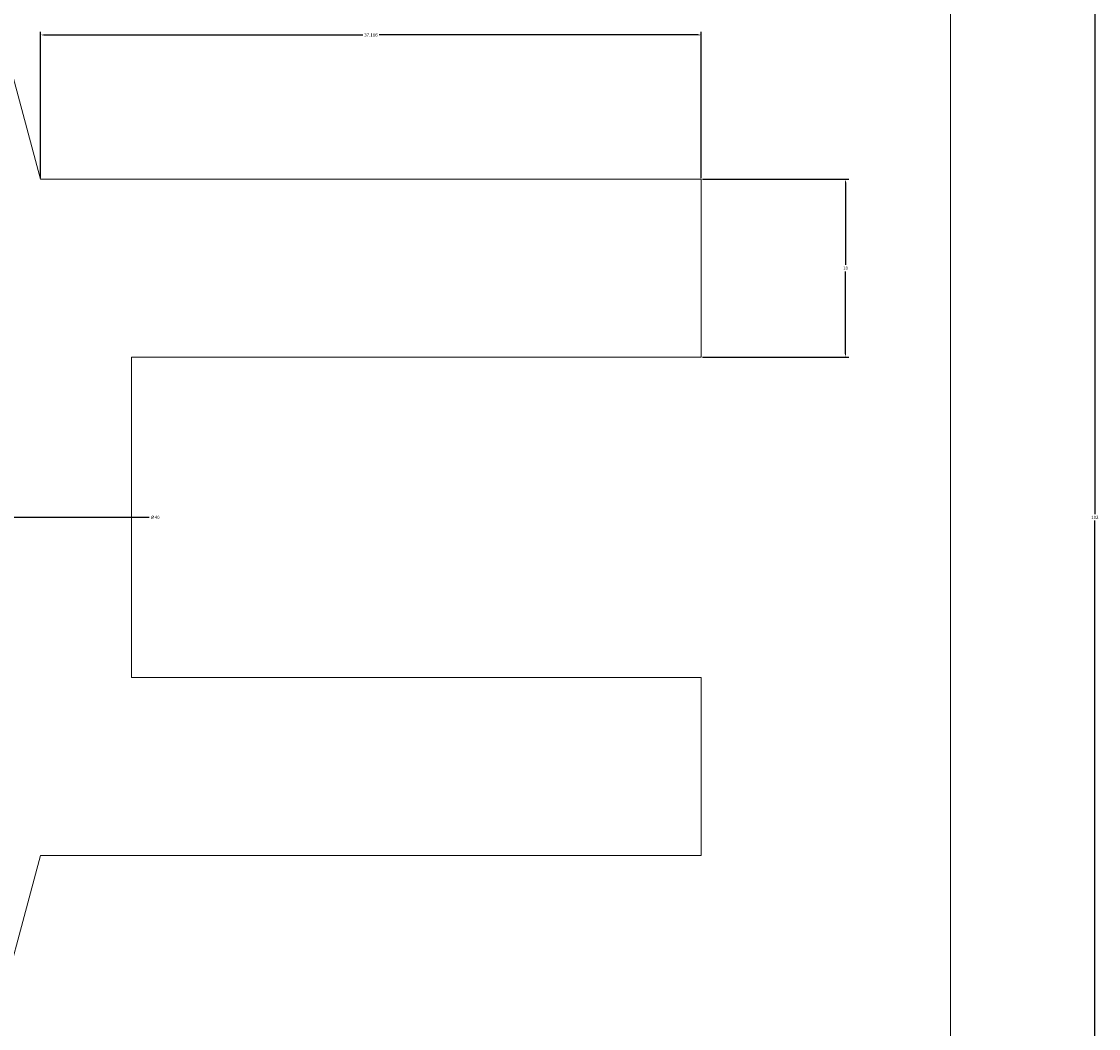
# Model space of a CAD drawing. Units: millimetres. Extents: x 2597 to 2768, y 1809 to 1980.
# Tile 6 of 7: x 2708 to 2768, y 1866 to 1922. Entities that reach past the tile are written whole.
import ezdxf

# ---------------------------------------------------------------- set-up
doc = ezdxf.new("R2010")
doc.units = ezdxf.units.MM
doc.layers.add('M-CONS', color=8, linetype='Continuous', lineweight=18)
doc.layers.add('M-DIMS', color=2, linetype='Continuous', lineweight=18)
doc.styles.get("Standard").update_dxf_attribs({"font": 'arial.ttf'})
doc.dimstyles.get("Standard").update_dxf_attribs({"dimtxt": 0.18, "dimasz": 0.18, "dimexe": 0.18, "dimexo": 0.0625, "dimgap": 0.09, "dimtad": 0, "dimtih": 1, "dimtoh": 1, "dimdec": 4, "dimzin": 0, "dimdsep": 46, "dimtxsty": 'Standard', "dimcen": 0.09, "dimadec": 0, "dimazin": 0, "dimtfac": 1, "dimtdec": 4, "dimtofl": 0, "dimtmove": 0, "dimatfit": 3, "dimfxl": 1, "dimtolj": 1, "dimtzin": 0, "dimarcsym": 0})

# ---------------------------------------------------------------- blocks, each defined once
blk = doc.blocks.new('*D6')
at = {"layer": 'Defpoints', "color": 0, "transparency": 16777216}
for p in [(2733.776, 1945.43), (2767.876, 1945.43), (2733.776, 1843.43)]:
    blk.add_point(p, dxfattribs=at)
at = {"layer": 'M-DIMS', "color": 0, "lineweight": -2, "transparency": 16777216}
for p, q in [((2733.838, 1945.43), (2768.056, 1945.43)), ((2767.876, 1945.25), (2767.876, 1894.612)), ((2767.876, 1843.61), (2767.876, 1894.248)), ((2733.838, 1843.43), (2768.056, 1843.43))]:
    blk.add_line(p, q, dxfattribs=at)
at = {"layer": 'M-DIMS', "color": 0, "transparency": 16777216}
for points in [[(2767.846, 1945.25), (2767.906, 1945.25), (2767.876, 1945.43)], [(2767.846, 1843.61), (2767.906, 1843.61), (2767.876, 1843.43)]]:
    blk.add_solid(points, dxfattribs=at)
at = {"layer": 'M-DIMS', "color": 0, "transparency": 16777216, "insert": (2767.876, 1894.43), "char_height": 0.18, "attachment_point": 5}
blk.add_mtext('\\A1;102', dxfattribs=at)
blk = doc.blocks.new('*D11')
at = {"layer": 'Defpoints', "color": 0, "transparency": 16777216}
for p in [(2745.776, 1913.43), (2745.776, 1903.43), (2753.876, 1903.43)]:
    blk.add_point(p, dxfattribs=at)
at = {"layer": 'M-DIMS', "color": 0, "lineweight": -2, "transparency": 16777216}
for p, q in [((2745.838, 1913.43), (2754.056, 1913.43)), ((2753.876, 1913.25), (2753.876, 1908.612)), ((2753.876, 1903.61), (2753.876, 1908.248)), ((2745.838, 1903.43), (2754.056, 1903.43))]:
    blk.add_line(p, q, dxfattribs=at)
at = {"layer": 'M-DIMS', "color": 0, "transparency": 16777216}
for points in [[(2753.846, 1913.25), (2753.906, 1913.25), (2753.876, 1913.43)], [(2753.846, 1903.61), (2753.906, 1903.61), (2753.876, 1903.43)]]:
    blk.add_solid(points, dxfattribs=at)
at = {"layer": 'M-DIMS', "color": 0, "transparency": 16777216, "insert": (2753.876, 1908.43), "char_height": 0.18, "attachment_point": 5}
blk.add_mtext('\\A1;10', dxfattribs=at)
blk = doc.blocks.new('*D12')
at = {"layer": 'Defpoints', "color": 0, "transparency": 16777216}
for p in [(2745.776, 1921.53), (2708.67, 1913.43), (2745.776, 1913.43)]:
    blk.add_point(p, dxfattribs=at)
at = {"layer": 'M-DIMS', "color": 0, "lineweight": -2, "transparency": 16777216}
for p, q in [((2708.67, 1913.493), (2708.67, 1921.71)), ((2708.85, 1921.53), (2726.759, 1921.53)), ((2745.596, 1921.53), (2727.686, 1921.53)), ((2745.776, 1913.493), (2745.776, 1921.71))]:
    blk.add_line(p, q, dxfattribs=at)
at = {"layer": 'M-DIMS', "color": 0, "transparency": 16777216}
for points in [[(2708.85, 1921.56), (2708.85, 1921.5), (2708.67, 1921.53)], [(2745.596, 1921.56), (2745.596, 1921.5), (2745.776, 1921.53)]]:
    blk.add_solid(points, dxfattribs=at)
at = {"layer": 'M-DIMS', "color": 0, "transparency": 16777216, "insert": (2727.223, 1921.53), "char_height": 0.18, "attachment_point": 5}
blk.add_mtext('\\A1;37.106', dxfattribs=at)
blk = doc.blocks.new('*D15')
at = {"layer": 'Defpoints', "color": 0, "transparency": 16777216}
for p in [(2662.776, 1894.43), (2702.776, 1894.43)]:
    blk.add_point(p, dxfattribs=at)
at = {"layer": 'M-DIMS', "color": 0, "lineweight": -2, "transparency": 16777216}
for p, q in [((2682.686, 1894.43), (2682.866, 1894.43)), ((2682.776, 1894.34), (2682.776, 1894.52)), ((2714.776, 1894.43), (2702.956, 1894.43))]:
    blk.add_line(p, q, dxfattribs=at)
at = {"layer": 'M-DIMS', "color": 0, "transparency": 16777216}
blk.add_solid([(2702.956, 1894.46), (2702.956, 1894.4), (2702.776, 1894.43)], dxfattribs=at)
at = {"layer": 'M-DIMS', "color": 0, "transparency": 16777216, "insert": (2715.092, 1894.43), "char_height": 0.18, "attachment_point": 5}
blk.add_mtext('\\A1;∅40', dxfattribs=at)

msp = doc.modelspace()

# ---------------------------------------------------------------- linework, layer by layer
at = {"layer": 'M-CONS', "extrusion": (0, -1, 0)}
msp.add_line((2708.6698, 1875.4301, 56), (2728.6698, 1875.4301, 56), dxfattribs=at)
at = {"layer": 'M-CONS'}
msp.add_lwpolyline([(2631.7756, 1817.4301), (2733.7756, 1817.4301, 0.4142136), (2759.7756, 1843.4301), (2759.7756, 1945.4301, 0.4142136), (2733.7756, 1971.4301), (2631.7756, 1971.4301, 0.4142136), (2605.7756, 1945.4301), (2605.7756, 1843.4301, 0.4142136)], format="xyb", close=True, dxfattribs=at)
msp.add_lwpolyline([(2713.7756, 1903.4301), (2745.7756, 1903.4301), (2745.7756, 1913.4301), (2708.6698, 1913.4301), (2700.1588, 1945.1014, 0.7667514), (2665.3923, 1945.1014), (2656.8814, 1913.4301), (2619.7756, 1913.4301), (2619.7756, 1903.4301), (2651.7756, 1903.4301), (2651.7756, 1885.4301), (2619.7756, 1885.4301), (2619.7756, 1875.4301), (2656.8814, 1875.4301), (2665.3923, 1843.7587, 0.7667514), (2700.1588, 1843.7587), (2708.6698, 1875.4301), (2745.7756, 1875.4301), (2745.7756, 1885.4301), (2713.7756, 1885.4301), (2713.7756, 1903.4301), (2713.7756, 1894.4301)], format="xyb", dxfattribs=at)
at = {"layer": 'M-CONS', "extrusion": (0, -1, 0)}
msp.add_circle((2728.6698, 44, -1875.4301), 5, dxfattribs=at)

# ---------------------------------------------------------------- dimensions: what is measured, and where the dimension line sits
at = {"layer": 'M-DIMS'}
for base, p1, p2, angle, picture, middle in [((2767.8756, 1945.4301), (2733.7756, 1843.4301), (2733.7756, 1945.4301), 90, '*D6', (2767.8756, 1894.4301)), ((2753.8756, 1903.4301), (2745.7756, 1913.4301), (2745.7756, 1903.4301), 270, '*D11', (2753.8756, 1908.4301))]:
    dim = msp.add_linear_dim(base=base, p1=p1, p2=p2, angle=angle, dimstyle='Standard', override={"dimdec": 0, "dimlfac": 1, "dimrnd": 0, "dimzin": 0, "dimdsep": 46, "dimlunit": 2}, dxfattribs=at)
    dim.commit()
    dim.dimension.update_dxf_attribs({"geometry": picture, "text_midpoint": middle})
dim = msp.add_linear_dim(base=(2745.7756, 1921.5301), p1=(2708.6698, 1913.4301), p2=(2745.7756, 1913.4301), dimstyle='Standard', override={"dimdec": 3, "dimlfac": 1, "dimrnd": 0, "dimzin": 0, "dimdsep": 46, "dimlunit": 2}, dxfattribs=at)
dim.commit()
dim.dimension.update_dxf_attribs({"geometry": '*D12', "text_midpoint": (2727.2227, 1921.5301)})
dim = msp.add_diameter_dim_2p(p1=(2662.7756, 1894.4302), p2=(2702.7756, 1894.43), dimstyle='Standard', override={"dimdec": 0, "dimlfac": 1, "dimrnd": 0, "dimzin": 0, "dimdsep": 46, "dimlunit": 2}, dxfattribs=at)
dim.commit()
dim.dimension.update_dxf_attribs({"geometry": '*D15', "text_midpoint": (2714.7756, 1894.4299), "dimtype": 163})

doc.saveas('drawing.dxf')
